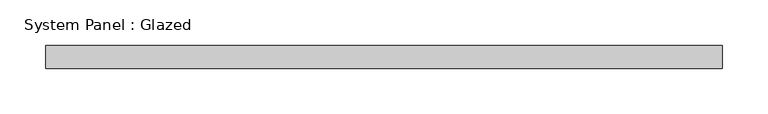
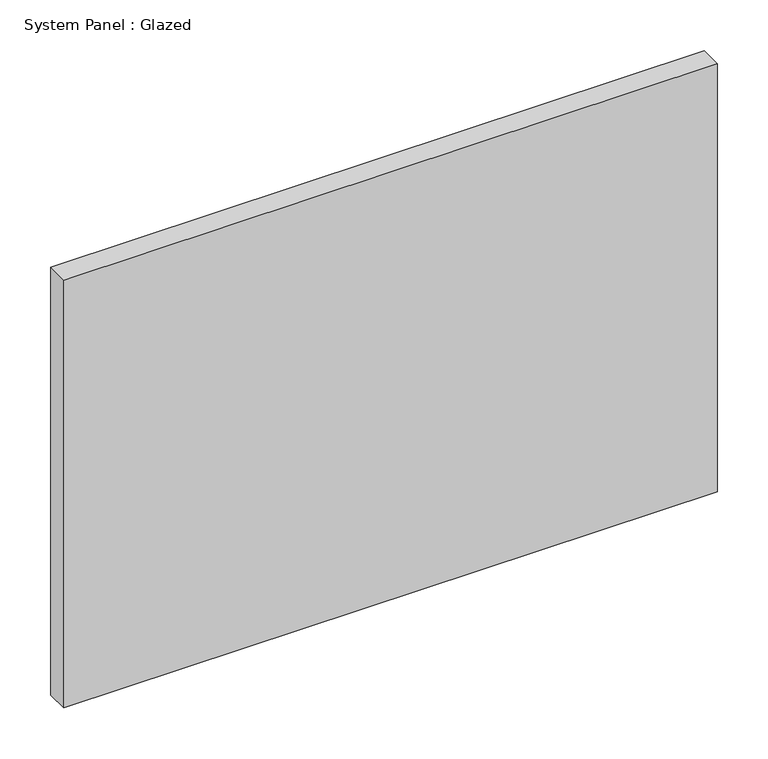
"""IFC4 building model written with IfcOpenShell, lengths in millimetres: plate geometry, System Panel : Glazed."""

from ifc_helpers import new_model, si_unit, origin, origin_with_axes, place, context, project, spatial, polyline, outline, extrude, source, transform, mapped, element, save


def system_panel_glazed_15008f27(model_context):
    return source(origin(), model_context, "Body", "SweptSolid", [
        extrude(outline(polyline([(371.475, -44.45), (-371.475, -44.45), (-371.475, -19.05), (371.475, -19.05), (371.475, -44.45)])), origin_with_axes(), (0.0, 0.0, 1.0), 514.35),
    ])


if __name__ == "__main__":
    model = new_model("IFC4")
    model_context = context("Model", 3, world=origin())
    ifc_project = project(units=[si_unit("LENGTHUNIT", "METRE", prefix="MILLI")], contexts=[model_context])
    site = spatial("IfcSite", under=ifc_project)
    building = spatial("IfcBuilding", under=site)
    placement = place(None, origin())
    system_panel_glazed_shape = system_panel_glazed_15008f27(model_context)
    element("IfcPlate", 1, ObjectType="System Panel : Glazed", at=placement, inside=building, context=model_context, shape_type="MappedRepresentation", body=[
        mapped(system_panel_glazed_shape, transform((0.0, 0.0, 0.0), x_axis=(1.0, 0.0, 0.0), y_axis=(0.0, 1.0, 0.0), z_axis=(0.0, 0.0, 1.0))),
    ])
    save(model, "model.ifc")

# Revit data of these elements
# Type "System Panel : Glazed"
#   Construction Type Id = "GSP4R"
#   Analytic Construction = "1/8 in Pilkington single glazing"
#   Visual Light Transmittance = 0.9
#   Solar Heat Gain Coefficient = 0.86
#   Heat Transfer Coefficient (U) = 1.18115 BTU/(h·ft²·°F)
#   Define Thermal Properties by = 1
# Element 1 (IfcPlate, "System Panel : Glazed")
#   Materials on its faces: "glass panel 223"
# Materials
#   "glass panel 223": class "Generic", colour RGB 120 120 120, transparency 0, Cost = 0
